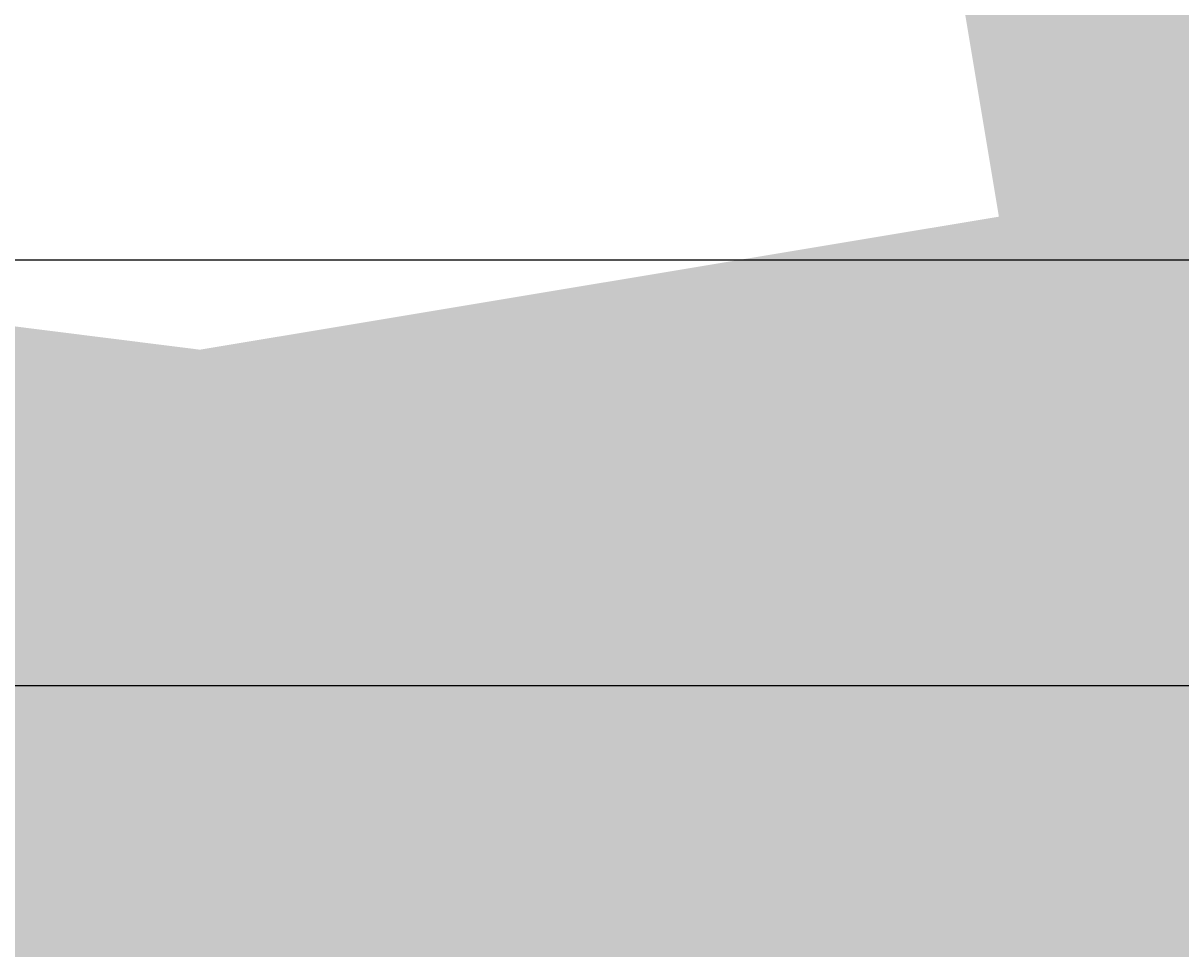
# Model space of a CAD drawing. Units: millimetres. Extents: x -22994 to 29398, y -19990 to 20176.
# Tile 120 of 135: x 245 to 296, y 124 to 165. Entities that reach past the tile are written whole.
import ezdxf

# ---------------------------------------------------------------- set-up
doc = ezdxf.new("R2010")
doc.units = ezdxf.units.MM
doc.header["$MEASUREMENT"] = 0
doc.layers.add('M-DIMS', color=2, linetype='Continuous', lineweight=18)
doc.styles.get("Standard").update_dxf_attribs({"font": 'arial.ttf'})
doc.dimstyles.get("Standard").update_dxf_attribs({"dimtxt": 0.18, "dimasz": 10000, "dimexe": 0.18, "dimexo": 0.0625, "dimgap": 0.09, "dimtad": 0, "dimtih": 1, "dimtoh": 1, "dimdec": 0, "dimzin": 0, "dimdsep": 46, "dimtxsty": 'Standard', "dimcen": 0.09, "dimadec": 0, "dimazin": 0, "dimtfac": 1, "dimtdec": 0, "dimtofl": 0, "dimtmove": 0, "dimatfit": 3, "dimfxl": 1, "dimtolj": 1, "dimtzin": 0, "dimlwd": 30, "dimarcsym": 0})

# ---------------------------------------------------------------- blocks, each defined once
blk = doc.blocks.new('*D2')
at = {"layer": 'Defpoints', "color": 0, "transparency": 16777216}
for p in [(6.677, 10.271), (290.852, 10.271), (290.852, -5.079)]:
    blk.add_point(p, dxfattribs=at)
at = {"layer": 'M-DIMS', "color": 0, "lineweight": -2, "transparency": 16777216}
for p, q in [((6.677, 10.209), (6.677, -5.259)), ((290.852, 10.209), (290.852, -5.259))]:
    blk.add_line(p, q, dxfattribs=at)
at = {"layer": 'M-DIMS', "color": 0, "lineweight": 30, "transparency": 16777216}
for p, q in [((-9993.323, -5.079), (-19993.323, -5.079)), ((10290.852, -5.079), (20290.852, -5.079))]:
    blk.add_line(p, q, dxfattribs=at)
at = {"layer": 'M-DIMS', "color": 0, "transparency": 16777216}
for points in [[(-9993.323, 1661.588), (-9993.323, -1671.745), (6.677, -5.079)], [(10290.852, 1661.588), (10290.852, -1671.745), (290.852, -5.079)]]:
    blk.add_solid(points, dxfattribs=at)
at = {"layer": 'M-DIMS', "color": 0, "transparency": 16777216, "insert": (148.765, -5.079), "char_height": 0.18, "attachment_point": 5}
blk.add_mtext('\\A1;284.2', dxfattribs=at)
blk = doc.blocks.new('*D3')
at = {"layer": 'Defpoints', "color": 0, "transparency": 16777216}
for p in [(110.265, 204.165), (110.265, 176.366), (95.833, 127.967)]:
    blk.add_point(p, dxfattribs=at)
at = {"layer": 'M-DIMS', "color": 0, "lineweight": 30, "transparency": 16777216}
for p, q in [((-9904.167, 204.165), (-19904.167, 204.165)), ((10110.265, 204.165), (20110.265, 204.165))]:
    blk.add_line(p, q, dxfattribs=at)
at = {"layer": 'M-DIMS', "color": 0, "lineweight": -2, "transparency": 16777216}
for p, q in [((95.833, 128.03), (95.833, 204.345)), ((110.265, 176.429), (110.265, 204.345))]:
    blk.add_line(p, q, dxfattribs=at)
at = {"layer": 'M-DIMS', "color": 0, "transparency": 16777216}
for points in [[(-9904.167, 1870.832), (-9904.167, -1462.501), (95.833, 204.165)], [(10110.265, 1870.832), (10110.265, -1462.501), (110.265, 204.165)]]:
    blk.add_solid(points, dxfattribs=at)
at = {"layer": 'M-DIMS', "color": 0, "transparency": 16777216, "insert": (103.049, 204.165), "char_height": 0.18, "attachment_point": 5}
blk.add_mtext('\\A1;14.432', dxfattribs=at)
blk = doc.blocks.new('*D4')
at = {"layer": 'Defpoints', "color": 0, "transparency": 16777216}
for p in [(116.265, 204.165), (110.265, 176.366), (116.265, 176.366)]:
    blk.add_point(p, dxfattribs=at)
at = {"layer": 'M-DIMS', "color": 0, "lineweight": 30, "transparency": 16777216}
for p, q in [((-9889.735, 204.165), (-19889.735, 204.165)), ((10116.265, 204.165), (20116.265, 204.165))]:
    blk.add_line(p, q, dxfattribs=at)
at = {"layer": 'M-DIMS', "color": 0, "lineweight": -2, "transparency": 16777216}
for p, q in [((110.265, 176.429), (110.265, 204.345)), ((116.265, 176.429), (116.265, 204.345))]:
    blk.add_line(p, q, dxfattribs=at)
at = {"layer": 'M-DIMS', "color": 0, "transparency": 16777216}
for points in [[(-9889.735, 1870.832), (-9889.735, -1462.501), (110.265, 204.165)], [(10116.265, 1870.832), (10116.265, -1462.501), (116.265, 204.165)]]:
    blk.add_solid(points, dxfattribs=at)
at = {"layer": 'M-DIMS', "color": 0, "transparency": 16777216, "insert": (113.265, 204.165), "char_height": 0.18, "attachment_point": 5}
blk.add_mtext('\\A1;6', dxfattribs=at)
blk = doc.blocks.new('*D5')
at = {"layer": 'Defpoints', "color": 0, "transparency": 16777216}
for p in [(181.265, 204.165), (116.265, 176.366), (181.265, 176.366)]:
    blk.add_point(p, dxfattribs=at)
at = {"layer": 'M-DIMS', "color": 0, "lineweight": 30, "transparency": 16777216}
for p, q in [((-9883.735, 204.165), (-19883.735, 204.165)), ((10181.265, 204.165), (20181.265, 204.165))]:
    blk.add_line(p, q, dxfattribs=at)
at = {"layer": 'M-DIMS', "color": 0, "lineweight": -2, "transparency": 16777216}
for p, q in [((116.265, 176.429), (116.265, 204.345)), ((181.265, 176.429), (181.265, 204.345))]:
    blk.add_line(p, q, dxfattribs=at)
at = {"layer": 'M-DIMS', "color": 0, "transparency": 16777216}
for points in [[(-9883.735, 1870.832), (-9883.735, -1462.501), (116.265, 204.165)], [(10181.265, 1870.832), (10181.265, -1462.501), (181.265, 204.165)]]:
    blk.add_solid(points, dxfattribs=at)
at = {"layer": 'M-DIMS', "color": 0, "transparency": 16777216, "insert": (148.765, 204.165), "char_height": 0.18, "attachment_point": 5}
blk.add_mtext('\\A1;65', dxfattribs=at)
blk = doc.blocks.new('*D6')
at = {"layer": 'Defpoints', "color": 0, "transparency": 16777216}
for p in [(187.265, 204.165), (181.265, 176.366), (187.265, 176.366)]:
    blk.add_point(p, dxfattribs=at)
at = {"layer": 'M-DIMS', "color": 0, "lineweight": 30, "transparency": 16777216}
for p, q in [((-9818.735, 204.165), (-19818.735, 204.165)), ((10187.265, 204.165), (20187.265, 204.165))]:
    blk.add_line(p, q, dxfattribs=at)
at = {"layer": 'M-DIMS', "color": 0, "lineweight": -2, "transparency": 16777216}
for p, q in [((181.265, 176.429), (181.265, 204.345)), ((187.265, 176.429), (187.265, 204.345))]:
    blk.add_line(p, q, dxfattribs=at)
at = {"layer": 'M-DIMS', "color": 0, "transparency": 16777216}
for points in [[(-9818.735, 1870.832), (-9818.735, -1462.501), (181.265, 204.165)], [(10187.265, 1870.832), (10187.265, -1462.501), (187.265, 204.165)]]:
    blk.add_solid(points, dxfattribs=at)
at = {"layer": 'M-DIMS', "color": 0, "transparency": 16777216, "insert": (184.265, 204.165), "char_height": 0.18, "attachment_point": 5}
blk.add_mtext('\\A1;6', dxfattribs=at)
blk = doc.blocks.new('*D7')
at = {"layer": 'Defpoints', "color": 0, "transparency": 16777216}
for p in [(201.697, 204.165), (187.265, 176.366), (201.697, 127.967)]:
    blk.add_point(p, dxfattribs=at)
at = {"layer": 'M-DIMS', "color": 0, "lineweight": 30, "transparency": 16777216}
for p, q in [((-9812.735, 204.165), (-19812.735, 204.165)), ((10201.697, 204.165), (20201.697, 204.165))]:
    blk.add_line(p, q, dxfattribs=at)
at = {"layer": 'M-DIMS', "color": 0, "lineweight": -2, "transparency": 16777216}
for p, q in [((187.265, 176.429), (187.265, 204.345)), ((201.697, 128.03), (201.697, 204.345))]:
    blk.add_line(p, q, dxfattribs=at)
at = {"layer": 'M-DIMS', "color": 0, "transparency": 16777216}
for points in [[(-9812.735, 1870.832), (-9812.735, -1462.501), (187.265, 204.165)], [(10201.697, 1870.832), (10201.697, -1462.501), (201.697, 204.165)]]:
    blk.add_solid(points, dxfattribs=at)
at = {"layer": 'M-DIMS', "color": 0, "transparency": 16777216, "insert": (194.481, 204.165), "char_height": 0.18, "attachment_point": 5}
blk.add_mtext('\\A1;14.432', dxfattribs=at)
blk = doc.blocks.new('*D8')
at = {"layer": 'Defpoints', "color": 0, "transparency": 16777216}
for p in [(227.648, 204.165), (227.648, 146.73), (201.697, 127.967)]:
    blk.add_point(p, dxfattribs=at)
at = {"layer": 'M-DIMS', "color": 0, "lineweight": 30, "transparency": 16777216}
for p, q in [((-9798.303, 204.165), (-19798.303, 204.165)), ((10227.648, 204.165), (20227.648, 204.165))]:
    blk.add_line(p, q, dxfattribs=at)
at = {"layer": 'M-DIMS', "color": 0, "lineweight": -2, "transparency": 16777216}
for p, q in [((201.697, 128.03), (201.697, 204.345)), ((227.648, 146.792), (227.648, 204.345))]:
    blk.add_line(p, q, dxfattribs=at)
at = {"layer": 'M-DIMS', "color": 0, "transparency": 16777216}
for points in [[(-9798.303, 1870.832), (-9798.303, -1462.501), (201.697, 204.165)], [(10227.648, 1870.832), (10227.648, -1462.501), (227.648, 204.165)]]:
    blk.add_solid(points, dxfattribs=at)
at = {"layer": 'M-DIMS', "color": 0, "transparency": 16777216, "insert": (214.673, 204.165), "char_height": 0.18, "attachment_point": 5}
blk.add_mtext('\\A1;25.95', dxfattribs=at)
blk = doc.blocks.new('*D9')
at = {"layer": 'Defpoints', "color": 0, "transparency": 16777216}
for p in [(187.265, 176.366), (306.202, 176.366), (290.852, 10.271)]:
    blk.add_point(p, dxfattribs=at)
at = {"layer": 'M-DIMS', "color": 0, "lineweight": 30, "transparency": 16777216}
for p, q in [((306.202, 10176.366), (306.202, 20176.366)), ((306.202, -9989.729), (306.202, -19989.729))]:
    blk.add_line(p, q, dxfattribs=at)
at = {"layer": 'M-DIMS', "color": 0, "lineweight": -2, "transparency": 16777216}
for p, q in [((187.327, 176.366), (306.382, 176.366)), ((290.915, 10.271), (306.382, 10.271))]:
    blk.add_line(p, q, dxfattribs=at)
at = {"layer": 'M-DIMS', "color": 0, "transparency": 16777216}
for points in [[(-1360.465, 10176.366), (1972.869, 10176.366), (306.202, 176.366)], [(-1360.465, -9989.729), (1972.869, -9989.729), (306.202, 10.271)]]:
    blk.add_solid(points, dxfattribs=at)
at = {"layer": 'M-DIMS', "color": 0, "transparency": 16777216, "insert": (306.202, 93.319), "char_height": 0.18, "attachment_point": 5}
blk.add_mtext('\\A1;166.1', dxfattribs=at)
blk = doc.blocks.new('*D10')
at = {"layer": 'Defpoints', "color": 0, "transparency": 16777216}
for p in [(125.65, 136.071), (133.346, 136.071), (133.346, -5.079)]:
    blk.add_point(p, dxfattribs=at)
at = {"layer": 'M-DIMS', "color": 0, "lineweight": -2, "transparency": 16777216}
for p, q in [((125.65, 136.009), (125.65, -5.259)), ((133.346, 136.009), (133.346, -5.259))]:
    blk.add_line(p, q, dxfattribs=at)
at = {"layer": 'M-DIMS', "color": 0, "lineweight": 30, "transparency": 16777216}
for p, q in [((-9874.35, -5.079), (-19874.35, -5.079)), ((10133.346, -5.079), (20133.346, -5.079))]:
    blk.add_line(p, q, dxfattribs=at)
at = {"layer": 'M-DIMS', "color": 0, "transparency": 16777216}
for points in [[(-9874.35, 1661.588), (-9874.35, -1671.745), (125.65, -5.079)], [(10133.346, 1661.588), (10133.346, -1671.745), (133.346, -5.079)]]:
    blk.add_solid(points, dxfattribs=at)
at = {"layer": 'M-DIMS', "color": 0, "transparency": 16777216, "insert": (129.498, -5.079), "char_height": 0.18, "attachment_point": 5}
blk.add_mtext('\\A1;7.696', dxfattribs=at)
blk = doc.blocks.new('*D11')
at = {"layer": 'Defpoints', "color": 0, "transparency": 16777216}
for p in [(133.346, 136.071), (135.65, 136.071), (135.65, -5.079)]:
    blk.add_point(p, dxfattribs=at)
at = {"layer": 'M-DIMS', "color": 0, "lineweight": -2, "transparency": 16777216}
for p, q in [((133.346, 136.009), (133.346, -5.259)), ((135.65, 136.009), (135.65, -5.259))]:
    blk.add_line(p, q, dxfattribs=at)
at = {"layer": 'M-DIMS', "color": 0, "lineweight": 30, "transparency": 16777216}
for p, q in [((-9866.654, -5.079), (-19866.654, -5.079)), ((10135.65, -5.079), (20135.65, -5.079))]:
    blk.add_line(p, q, dxfattribs=at)
at = {"layer": 'M-DIMS', "color": 0, "transparency": 16777216}
for points in [[(-9866.654, 1661.588), (-9866.654, -1671.745), (133.346, -5.079)], [(10135.65, 1661.588), (10135.65, -1671.745), (135.65, -5.079)]]:
    blk.add_solid(points, dxfattribs=at)
at = {"layer": 'M-DIMS', "color": 0, "transparency": 16777216, "insert": (134.498, -5.079), "char_height": 0.18, "attachment_point": 5}
blk.add_mtext('\\A1;2.304', dxfattribs=at)
blk = doc.blocks.new('*D12')
at = {"layer": 'Defpoints', "color": 0, "transparency": 16777216}
for p in [(135.65, 136.071), (145.65, 136.071), (145.65, -5.079)]:
    blk.add_point(p, dxfattribs=at)
at = {"layer": 'M-DIMS', "color": 0, "lineweight": -2, "transparency": 16777216}
for p, q in [((135.65, 136.009), (135.65, -5.259)), ((145.65, 136.009), (145.65, -5.259))]:
    blk.add_line(p, q, dxfattribs=at)
at = {"layer": 'M-DIMS', "color": 0, "lineweight": 30, "transparency": 16777216}
for p, q in [((-9864.35, -5.079), (-19864.35, -5.079)), ((10145.65, -5.079), (20145.65, -5.079))]:
    blk.add_line(p, q, dxfattribs=at)
at = {"layer": 'M-DIMS', "color": 0, "transparency": 16777216}
for points in [[(-9864.35, 1661.588), (-9864.35, -1671.745), (135.65, -5.079)], [(10145.65, 1661.588), (10145.65, -1671.745), (145.65, -5.079)]]:
    blk.add_solid(points, dxfattribs=at)
at = {"layer": 'M-DIMS', "color": 0, "transparency": 16777216, "insert": (140.65, -5.079), "char_height": 0.18, "attachment_point": 5}
blk.add_mtext('\\A1;10', dxfattribs=at)
blk = doc.blocks.new('*D13')
at = {"layer": 'Defpoints', "color": 0, "transparency": 16777216}
for p in [(145.65, 136.071), (155.65, 136.071), (155.65, -5.079)]:
    blk.add_point(p, dxfattribs=at)
at = {"layer": 'M-DIMS', "color": 0, "lineweight": -2, "transparency": 16777216}
for p, q in [((145.65, 136.009), (145.65, -5.259)), ((155.65, 136.009), (155.65, -5.259))]:
    blk.add_line(p, q, dxfattribs=at)
at = {"layer": 'M-DIMS', "color": 0, "lineweight": 30, "transparency": 16777216}
for p, q in [((-9854.35, -5.079), (-19854.35, -5.079)), ((10155.65, -5.079), (20155.65, -5.079))]:
    blk.add_line(p, q, dxfattribs=at)
at = {"layer": 'M-DIMS', "color": 0, "transparency": 16777216}
for points in [[(-9854.35, 1661.588), (-9854.35, -1671.745), (145.65, -5.079)], [(10155.65, 1661.588), (10155.65, -1671.745), (155.65, -5.079)]]:
    blk.add_solid(points, dxfattribs=at)
at = {"layer": 'M-DIMS', "color": 0, "transparency": 16777216, "insert": (150.65, -5.079), "char_height": 0.18, "attachment_point": 5}
blk.add_mtext('\\A1;10', dxfattribs=at)
blk = doc.blocks.new('*D14')
at = {"layer": 'Defpoints', "color": 0, "transparency": 16777216}
for p in [(155.65, 136.071), (165.65, 136.071), (165.65, -5.079)]:
    blk.add_point(p, dxfattribs=at)
at = {"layer": 'M-DIMS', "color": 0, "lineweight": -2, "transparency": 16777216}
for p, q in [((155.65, 136.009), (155.65, -5.259)), ((165.65, 136.009), (165.65, -5.259))]:
    blk.add_line(p, q, dxfattribs=at)
at = {"layer": 'M-DIMS', "color": 0, "lineweight": 30, "transparency": 16777216}
for p, q in [((-9844.35, -5.079), (-19844.35, -5.079)), ((10165.65, -5.079), (20165.65, -5.079))]:
    blk.add_line(p, q, dxfattribs=at)
at = {"layer": 'M-DIMS', "color": 0, "transparency": 16777216}
for points in [[(-9844.35, 1661.588), (-9844.35, -1671.745), (155.65, -5.079)], [(10165.65, 1661.588), (10165.65, -1671.745), (165.65, -5.079)]]:
    blk.add_solid(points, dxfattribs=at)
at = {"layer": 'M-DIMS', "color": 0, "transparency": 16777216, "insert": (160.65, -5.079), "char_height": 0.18, "attachment_point": 5}
blk.add_mtext('\\A1;10', dxfattribs=at)
blk = doc.blocks.new('*D15')
at = {"layer": 'Defpoints', "color": 0, "transparency": 16777216}
for p in [(173.346, 154.788), (173.346, 136.071), (306.202, 136.071)]:
    blk.add_point(p, dxfattribs=at)
at = {"layer": 'M-DIMS', "color": 0, "lineweight": 30, "transparency": 16777216}
for p, q in [((306.202, 10154.788), (306.202, 20154.788)), ((306.202, -9863.929), (306.202, -19863.929))]:
    blk.add_line(p, q, dxfattribs=at)
at = {"layer": 'M-DIMS', "color": 0, "lineweight": -2, "transparency": 16777216}
for p, q in [((173.408, 154.788), (306.382, 154.788)), ((173.408, 136.071), (306.382, 136.071))]:
    blk.add_line(p, q, dxfattribs=at)
at = {"layer": 'M-DIMS', "color": 0, "transparency": 16777216}
for points in [[(-1360.465, 10154.788), (1972.869, 10154.788), (306.202, 154.788)], [(-1360.465, -9863.929), (1972.869, -9863.929), (306.202, 136.071)]]:
    blk.add_solid(points, dxfattribs=at)
at = {"layer": 'M-DIMS', "color": 0, "transparency": 16777216, "insert": (306.202, 145.43), "char_height": 0.18, "attachment_point": 5}
blk.add_mtext('\\A1;18.717', dxfattribs=at)
blk = doc.blocks.new('*D16')
at = {"layer": 'Defpoints', "color": 0, "transparency": 16777216}
for p in [(120.17, 204.165), (110.466, 48.035), (120.17, 48.035)]:
    blk.add_point(p, dxfattribs=at)
at = {"layer": 'M-DIMS', "color": 0, "lineweight": 30, "transparency": 16777216}
for p, q in [((-9889.534, 204.165), (-19889.534, 204.165)), ((10120.17, 204.165), (20120.17, 204.165))]:
    blk.add_line(p, q, dxfattribs=at)
at = {"layer": 'M-DIMS', "color": 0, "lineweight": -2, "transparency": 16777216}
for p, q in [((110.466, 48.097), (110.466, 204.345)), ((120.17, 48.097), (120.17, 204.345))]:
    blk.add_line(p, q, dxfattribs=at)
at = {"layer": 'M-DIMS', "color": 0, "transparency": 16777216}
for points in [[(-9889.534, 1870.832), (-9889.534, -1462.501), (110.466, 204.165)], [(10120.17, 1870.832), (10120.17, -1462.501), (120.17, 204.165)]]:
    blk.add_solid(points, dxfattribs=at)
at = {"layer": 'M-DIMS', "color": 0, "transparency": 16777216, "insert": (115.318, 204.165), "char_height": 0.18, "attachment_point": 5}
blk.add_mtext('\\A1;9.704', dxfattribs=at)
blk = doc.blocks.new('*D17')
at = {"layer": 'Defpoints', "color": 0, "transparency": 16777216}
for p in [(126.17, 204.165), (120.17, 48.035), (126.17, 48.035)]:
    blk.add_point(p, dxfattribs=at)
at = {"layer": 'M-DIMS', "color": 0, "lineweight": 30, "transparency": 16777216}
for p, q in [((-9879.83, 204.165), (-19879.83, 204.165)), ((10126.17, 204.165), (20126.17, 204.165))]:
    blk.add_line(p, q, dxfattribs=at)
at = {"layer": 'M-DIMS', "color": 0, "lineweight": -2, "transparency": 16777216}
for p, q in [((120.17, 48.097), (120.17, 204.345)), ((126.17, 48.097), (126.17, 204.345))]:
    blk.add_line(p, q, dxfattribs=at)
at = {"layer": 'M-DIMS', "color": 0, "transparency": 16777216}
for points in [[(-9879.83, 1870.832), (-9879.83, -1462.501), (120.17, 204.165)], [(10126.17, 1870.832), (10126.17, -1462.501), (126.17, 204.165)]]:
    blk.add_solid(points, dxfattribs=at)
at = {"layer": 'M-DIMS', "color": 0, "transparency": 16777216, "insert": (123.17, 204.165), "char_height": 0.18, "attachment_point": 5}
blk.add_mtext('\\A1;6', dxfattribs=at)
blk = doc.blocks.new('*D18')
at = {"layer": 'Defpoints', "color": 0, "transparency": 16777216}
for p in [(132.17, 204.165), (126.17, 48.035), (132.17, 48.035)]:
    blk.add_point(p, dxfattribs=at)
at = {"layer": 'M-DIMS', "color": 0, "lineweight": 30, "transparency": 16777216}
for p, q in [((-9873.83, 204.165), (-19873.83, 204.165)), ((10132.17, 204.165), (20132.17, 204.165))]:
    blk.add_line(p, q, dxfattribs=at)
at = {"layer": 'M-DIMS', "color": 0, "lineweight": -2, "transparency": 16777216}
for p, q in [((126.17, 48.097), (126.17, 204.345)), ((132.17, 48.097), (132.17, 204.345))]:
    blk.add_line(p, q, dxfattribs=at)
at = {"layer": 'M-DIMS', "color": 0, "transparency": 16777216}
for points in [[(-9873.83, 1870.832), (-9873.83, -1462.501), (126.17, 204.165)], [(10132.17, 1870.832), (10132.17, -1462.501), (132.17, 204.165)]]:
    blk.add_solid(points, dxfattribs=at)
at = {"layer": 'M-DIMS', "color": 0, "transparency": 16777216, "insert": (129.17, 204.165), "char_height": 0.18, "attachment_point": 5}
blk.add_mtext('\\A1;6', dxfattribs=at)
blk = doc.blocks.new('*D19')
at = {"layer": 'Defpoints', "color": 0, "transparency": 16777216}
for p in [(138.17, 204.165), (132.17, 48.035), (138.17, 48.035)]:
    blk.add_point(p, dxfattribs=at)
at = {"layer": 'M-DIMS', "color": 0, "lineweight": 30, "transparency": 16777216}
for p, q in [((-9867.83, 204.165), (-19867.83, 204.165)), ((10138.17, 204.165), (20138.17, 204.165))]:
    blk.add_line(p, q, dxfattribs=at)
at = {"layer": 'M-DIMS', "color": 0, "lineweight": -2, "transparency": 16777216}
for p, q in [((132.17, 48.097), (132.17, 204.345)), ((138.17, 48.097), (138.17, 204.345))]:
    blk.add_line(p, q, dxfattribs=at)
at = {"layer": 'M-DIMS', "color": 0, "transparency": 16777216}
for points in [[(-9867.83, 1870.832), (-9867.83, -1462.501), (132.17, 204.165)], [(10138.17, 1870.832), (10138.17, -1462.501), (138.17, 204.165)]]:
    blk.add_solid(points, dxfattribs=at)
at = {"layer": 'M-DIMS', "color": 0, "transparency": 16777216, "insert": (135.17, 204.165), "char_height": 0.18, "attachment_point": 5}
blk.add_mtext('\\A1;6', dxfattribs=at)
blk = doc.blocks.new('*D20')
at = {"layer": 'Defpoints', "color": 0, "transparency": 16777216}
for p in [(144.17, 204.165), (138.17, 48.035), (144.17, 48.035)]:
    blk.add_point(p, dxfattribs=at)
at = {"layer": 'M-DIMS', "color": 0, "lineweight": 30, "transparency": 16777216}
for p, q in [((-9861.83, 204.165), (-19861.83, 204.165)), ((10144.17, 204.165), (20144.17, 204.165))]:
    blk.add_line(p, q, dxfattribs=at)
at = {"layer": 'M-DIMS', "color": 0, "lineweight": -2, "transparency": 16777216}
for p, q in [((138.17, 48.097), (138.17, 204.345)), ((144.17, 48.097), (144.17, 204.345))]:
    blk.add_line(p, q, dxfattribs=at)
at = {"layer": 'M-DIMS', "color": 0, "transparency": 16777216}
for points in [[(-9861.83, 1870.832), (-9861.83, -1462.501), (138.17, 204.165)], [(10144.17, 1870.832), (10144.17, -1462.501), (144.17, 204.165)]]:
    blk.add_solid(points, dxfattribs=at)
at = {"layer": 'M-DIMS', "color": 0, "transparency": 16777216, "insert": (141.17, 204.165), "char_height": 0.18, "attachment_point": 5}
blk.add_mtext('\\A1;6', dxfattribs=at)
blk = doc.blocks.new('*D21')
at = {"layer": 'Defpoints', "color": 0, "transparency": 16777216}
for p in [(149.116, 204.165), (144.17, 48.035), (149.116, 48.035)]:
    blk.add_point(p, dxfattribs=at)
at = {"layer": 'M-DIMS', "color": 0, "lineweight": 30, "transparency": 16777216}
for p, q in [((-9855.83, 204.165), (-19855.83, 204.165)), ((10149.116, 204.165), (20149.116, 204.165))]:
    blk.add_line(p, q, dxfattribs=at)
at = {"layer": 'M-DIMS', "color": 0, "lineweight": -2, "transparency": 16777216}
for p, q in [((144.17, 48.097), (144.17, 204.345)), ((149.116, 48.097), (149.116, 204.345))]:
    blk.add_line(p, q, dxfattribs=at)
at = {"layer": 'M-DIMS', "color": 0, "transparency": 16777216}
for points in [[(-9855.83, 1870.832), (-9855.83, -1462.501), (144.17, 204.165)], [(10149.116, 1870.832), (10149.116, -1462.501), (149.116, 204.165)]]:
    blk.add_solid(points, dxfattribs=at)
at = {"layer": 'M-DIMS', "color": 0, "transparency": 16777216, "insert": (146.643, 204.165), "char_height": 0.18, "attachment_point": 5}
blk.add_mtext('\\A1;4.945', dxfattribs=at)
blk = doc.blocks.new('*D22')
at = {"layer": 'Defpoints', "color": 0, "transparency": 16777216}
for p in [(149.116, 30.99), (155.116, 30.99), (155.116, -5.079)]:
    blk.add_point(p, dxfattribs=at)
at = {"layer": 'M-DIMS', "color": 0, "lineweight": -2, "transparency": 16777216}
for p, q in [((149.116, 30.927), (149.116, -5.259)), ((155.116, 30.927), (155.116, -5.259))]:
    blk.add_line(p, q, dxfattribs=at)
at = {"layer": 'M-DIMS', "color": 0, "lineweight": 30, "transparency": 16777216}
for p, q in [((-9850.884, -5.079), (-19850.884, -5.079)), ((10155.116, -5.079), (20155.116, -5.079))]:
    blk.add_line(p, q, dxfattribs=at)
at = {"layer": 'M-DIMS', "color": 0, "transparency": 16777216}
for points in [[(-9850.884, 1661.588), (-9850.884, -1671.745), (149.116, -5.079)], [(10155.116, 1661.588), (10155.116, -1671.745), (155.116, -5.079)]]:
    blk.add_solid(points, dxfattribs=at)
at = {"layer": 'M-DIMS', "color": 0, "transparency": 16777216, "insert": (152.116, -5.079), "char_height": 0.18, "attachment_point": 5}
blk.add_mtext('\\A1;6', dxfattribs=at)
blk = doc.blocks.new('*D23')
at = {"layer": 'Defpoints', "color": 0, "transparency": 16777216}
for p in [(155.116, 30.99), (161.116, 30.99), (161.116, -5.079)]:
    blk.add_point(p, dxfattribs=at)
at = {"layer": 'M-DIMS', "color": 0, "lineweight": -2, "transparency": 16777216}
for p, q in [((155.116, 30.927), (155.116, -5.259)), ((161.116, 30.927), (161.116, -5.259))]:
    blk.add_line(p, q, dxfattribs=at)
at = {"layer": 'M-DIMS', "color": 0, "lineweight": 30, "transparency": 16777216}
for p, q in [((-9844.884, -5.079), (-19844.884, -5.079)), ((10161.116, -5.079), (20161.116, -5.079))]:
    blk.add_line(p, q, dxfattribs=at)
at = {"layer": 'M-DIMS', "color": 0, "transparency": 16777216}
for points in [[(-9844.884, 1661.588), (-9844.884, -1671.745), (155.116, -5.079)], [(10161.116, 1661.588), (10161.116, -1671.745), (161.116, -5.079)]]:
    blk.add_solid(points, dxfattribs=at)
at = {"layer": 'M-DIMS', "color": 0, "transparency": 16777216, "insert": (158.116, -5.079), "char_height": 0.18, "attachment_point": 5}
blk.add_mtext('\\A1;6', dxfattribs=at)
blk = doc.blocks.new('*D24')
at = {"layer": 'Defpoints', "color": 0, "transparency": 16777216}
for p in [(161.116, 30.99), (166.439, 30.99), (166.439, -5.079)]:
    blk.add_point(p, dxfattribs=at)
at = {"layer": 'M-DIMS', "color": 0, "lineweight": -2, "transparency": 16777216}
for p, q in [((161.116, 30.927), (161.116, -5.259)), ((166.439, 30.927), (166.439, -5.259))]:
    blk.add_line(p, q, dxfattribs=at)
at = {"layer": 'M-DIMS', "color": 0, "lineweight": 30, "transparency": 16777216}
for p, q in [((-9838.884, -5.079), (-19838.884, -5.079)), ((10166.439, -5.079), (20166.439, -5.079))]:
    blk.add_line(p, q, dxfattribs=at)
at = {"layer": 'M-DIMS', "color": 0, "transparency": 16777216}
for points in [[(-9838.884, 1661.588), (-9838.884, -1671.745), (161.116, -5.079)], [(10166.439, 1661.588), (10166.439, -1671.745), (166.439, -5.079)]]:
    blk.add_solid(points, dxfattribs=at)
at = {"layer": 'M-DIMS', "color": 0, "transparency": 16777216, "insert": (163.777, -5.079), "char_height": 0.18, "attachment_point": 5}
blk.add_mtext('\\A1;5.323', dxfattribs=at)
blk = doc.blocks.new('*D25')
at = {"layer": 'Defpoints', "color": 0, "transparency": 16777216}
for p in [(166.439, 30.99), (172.439, 30.99), (172.439, -5.079)]:
    blk.add_point(p, dxfattribs=at)
at = {"layer": 'M-DIMS', "color": 0, "lineweight": -2, "transparency": 16777216}
for p, q in [((166.439, 30.927), (166.439, -5.259)), ((172.439, 30.927), (172.439, -5.259))]:
    blk.add_line(p, q, dxfattribs=at)
at = {"layer": 'M-DIMS', "color": 0, "lineweight": 30, "transparency": 16777216}
for p, q in [((-9833.561, -5.079), (-19833.561, -5.079)), ((10172.439, -5.079), (20172.439, -5.079))]:
    blk.add_line(p, q, dxfattribs=at)
at = {"layer": 'M-DIMS', "color": 0, "transparency": 16777216}
for points in [[(-9833.561, 1661.588), (-9833.561, -1671.745), (166.439, -5.079)], [(10172.439, 1661.588), (10172.439, -1671.745), (172.439, -5.079)]]:
    blk.add_solid(points, dxfattribs=at)
at = {"layer": 'M-DIMS', "color": 0, "transparency": 16777216, "insert": (169.439, -5.079), "char_height": 0.18, "attachment_point": 5}
blk.add_mtext('\\A1;6', dxfattribs=at)
blk = doc.blocks.new('*D26')
at = {"layer": 'Defpoints', "color": 0, "transparency": 16777216}
for p in [(172.439, 30.99), (178.439, 30.99), (178.439, -5.079)]:
    blk.add_point(p, dxfattribs=at)
at = {"layer": 'M-DIMS', "color": 0, "lineweight": -2, "transparency": 16777216}
for p, q in [((172.439, 30.927), (172.439, -5.259)), ((178.439, 30.927), (178.439, -5.259))]:
    blk.add_line(p, q, dxfattribs=at)
at = {"layer": 'M-DIMS', "color": 0, "lineweight": 30, "transparency": 16777216}
for p, q in [((-9827.561, -5.079), (-19827.561, -5.079)), ((10178.439, -5.079), (20178.439, -5.079))]:
    blk.add_line(p, q, dxfattribs=at)
at = {"layer": 'M-DIMS', "color": 0, "transparency": 16777216}
for points in [[(-9827.561, 1661.588), (-9827.561, -1671.745), (172.439, -5.079)], [(10178.439, 1661.588), (10178.439, -1671.745), (178.439, -5.079)]]:
    blk.add_solid(points, dxfattribs=at)
at = {"layer": 'M-DIMS', "color": 0, "transparency": 16777216, "insert": (175.439, -5.079), "char_height": 0.18, "attachment_point": 5}
blk.add_mtext('\\A1;6', dxfattribs=at)
blk = doc.blocks.new('*D27')
at = {"layer": 'Defpoints', "color": 0, "transparency": 16777216}
for p in [(178.439, 30.99), (188.117, 30.99), (188.117, -5.079)]:
    blk.add_point(p, dxfattribs=at)
at = {"layer": 'M-DIMS', "color": 0, "lineweight": -2, "transparency": 16777216}
for p, q in [((178.439, 30.927), (178.439, -5.259)), ((188.117, 30.927), (188.117, -5.259))]:
    blk.add_line(p, q, dxfattribs=at)
at = {"layer": 'M-DIMS', "color": 0, "lineweight": 30, "transparency": 16777216}
for p, q in [((-9821.561, -5.079), (-19821.561, -5.079)), ((10188.117, -5.079), (20188.117, -5.079))]:
    blk.add_line(p, q, dxfattribs=at)
at = {"layer": 'M-DIMS', "color": 0, "transparency": 16777216}
for points in [[(-9821.561, 1661.588), (-9821.561, -1671.745), (178.439, -5.079)], [(10188.117, 1661.588), (10188.117, -1671.745), (188.117, -5.079)]]:
    blk.add_solid(points, dxfattribs=at)
at = {"layer": 'M-DIMS', "color": 0, "transparency": 16777216, "insert": (183.278, -5.079), "char_height": 0.18, "attachment_point": 5}
blk.add_mtext('\\A1;9.679', dxfattribs=at)
blk = doc.blocks.new('*D28')
at = {"layer": 'Defpoints', "color": 0, "transparency": 16777216}
for p in [(188.117, 48.035), (306.202, 48.035), (188.117, 30.99)]:
    blk.add_point(p, dxfattribs=at)
at = {"layer": 'M-DIMS', "color": 0, "lineweight": 30, "transparency": 16777216}
for p, q in [((306.202, 10048.035), (306.202, 20048.035)), ((306.202, -9969.01), (306.202, -19969.01))]:
    blk.add_line(p, q, dxfattribs=at)
at = {"layer": 'M-DIMS', "color": 0, "lineweight": -2, "transparency": 16777216}
for p, q in [((188.18, 48.035), (306.382, 48.035)), ((188.18, 30.99), (306.382, 30.99))]:
    blk.add_line(p, q, dxfattribs=at)
at = {"layer": 'M-DIMS', "color": 0, "transparency": 16777216}
for points in [[(-1360.465, 10048.035), (1972.869, 10048.035), (306.202, 48.035)], [(-1360.465, -9969.01), (1972.869, -9969.01), (306.202, 30.99)]]:
    blk.add_solid(points, dxfattribs=at)
at = {"layer": 'M-DIMS', "color": 0, "transparency": 16777216, "insert": (306.202, 39.512), "char_height": 0.18, "attachment_point": 5}
blk.add_mtext('\\A1;17.045', dxfattribs=at)
blk = doc.blocks.new('*D29')
at = {"layer": 'Defpoints', "color": 0, "transparency": 16777216}
for p in [(36.801, 80.045), (64.03, 80.045)]:
    blk.add_point(p, dxfattribs=at)
at = {"layer": 'M-DIMS', "color": 0, "lineweight": -2, "transparency": 16777216}
for p, q in [((50.325, 80.045), (50.505, 80.045)), ((50.415, 79.955), (50.415, 80.135))]:
    blk.add_line(p, q, dxfattribs=at)
at = {"layer": 'M-DIMS', "color": 0, "lineweight": 30, "transparency": 16777216}
blk.add_line((20064.03, 80.03), (10064.03, 80.038), dxfattribs=at)
at = {"layer": 'M-DIMS', "color": 0, "transparency": 16777216}
blk.add_solid([(10064.031, 1746.704), (10064.028, -1586.629), (64.03, 80.045)], dxfattribs=at)
at = {"layer": 'M-DIMS', "color": 0, "transparency": 16777216, "insert": (20064.521, 80.03), "char_height": 0.18, "attachment_point": 5}
blk.add_mtext('\\A1;∅27.23', dxfattribs=at)
blk = doc.blocks.new('*D30')
at = {"layer": 'Defpoints', "color": 0, "transparency": 16777216}
for p in [(216.315, 146.729), (238.982, 146.73)]:
    blk.add_point(p, dxfattribs=at)
at = {"layer": 'M-DIMS', "color": 0, "lineweight": 30, "transparency": 16777216}
blk.add_line((20238.982, 147.496), (10238.982, 147.113), dxfattribs=at)
at = {"layer": 'M-DIMS', "color": 0, "lineweight": -2, "transparency": 16777216}
for p, q in [((227.558, 146.73), (227.738, 146.73)), ((227.648, 146.64), (227.648, 146.82))]:
    blk.add_line(p, q, dxfattribs=at)
at = {"layer": 'M-DIMS', "color": 0, "transparency": 16777216}
blk.add_solid([(10238.918, 1813.78), (10239.046, -1519.554), (238.982, 146.73)], dxfattribs=at)
at = {"layer": 'M-DIMS', "color": 0, "transparency": 16777216, "insert": (20239.544, 147.496), "char_height": 0.18, "attachment_point": 5}
blk.add_mtext('\\A1;∅22.667', dxfattribs=at)
blk = doc.blocks.new('*D31')
at = {"layer": 'Defpoints', "color": 0, "transparency": 16777216}
for p in [(223.164, 146.729), (232.133, 146.73)]:
    blk.add_point(p, dxfattribs=at)
at = {"layer": 'M-DIMS', "color": 0, "lineweight": 30, "transparency": 16777216}
blk.add_line((20232.133, 148.666), (10232.133, 147.698), dxfattribs=at)
at = {"layer": 'M-DIMS', "color": 0, "lineweight": -2, "transparency": 16777216}
for p, q in [((227.558, 146.73), (227.738, 146.73)), ((227.648, 146.64), (227.648, 146.82))]:
    blk.add_line(p, q, dxfattribs=at)
at = {"layer": 'M-DIMS', "color": 0, "transparency": 16777216}
blk.add_solid([(10231.971, 1814.364), (10232.294, -1518.969), (232.133, 146.73)], dxfattribs=at)
at = {"layer": 'M-DIMS', "color": 0, "transparency": 16777216, "insert": (20232.625, 148.666), "char_height": 0.18, "attachment_point": 5}
blk.add_mtext('\\A1;∅8.969', dxfattribs=at)
blk = doc.blocks.new('*D33')
at = {"layer": 'Defpoints', "color": 0, "transparency": 16777216}
for p in [(229.561, 154.377), (232.997, 153.351)]:
    blk.add_point(p, dxfattribs=at)
at = {"layer": 'M-DIMS', "color": 0, "lineweight": -2, "transparency": 16777216}
for p, q in [((229.471, 154.377), (229.651, 154.377)), ((229.561, 154.287), (229.561, 154.467))]:
    blk.add_line(p, q, dxfattribs=at)
at = {"layer": 'M-DIMS', "color": 0, "lineweight": 30, "transparency": 16777216}
for p, q in [((19396.339, -5570.838), (9814.668, -2708.743)), ((29396.339, -5570.838), (19396.339, -5570.838))]:
    blk.add_line(p, q, dxfattribs=at)
at = {"layer": 'M-DIMS', "color": 0, "transparency": 16777216}
blk.add_solid([(10291.684, -1111.798), (9337.652, -4305.689), (232.997, 153.351)], dxfattribs=at)
at = {"layer": 'M-DIMS', "color": 0, "transparency": 16777216, "insert": (29397.012, -5570.838), "char_height": 0.18, "attachment_point": 5}
blk.add_mtext('\\A1;6X R3.586', dxfattribs=at)
blk = doc.blocks.new('*D34')
at = {"layer": 'Defpoints', "color": 0, "transparency": 16777216}
for p in [(178.58, 122.895), (176.812, 121.128)]:
    blk.add_point(p, dxfattribs=at)
at = {"layer": 'M-DIMS', "color": 0, "lineweight": 30, "transparency": 16777216}
for p, q in [((14322.436, 14263.311), (7250.508, 7193.103)), ((24322.436, 14263.311), (14322.436, 14263.311))]:
    blk.add_line(p, q, dxfattribs=at)
at = {"layer": 'M-DIMS', "color": 0, "lineweight": -2, "transparency": 16777216}
for p, q in [((176.722, 121.128), (176.902, 121.128)), ((176.812, 121.038), (176.812, 121.218))]:
    blk.add_line(p, q, dxfattribs=at)
at = {"layer": 'M-DIMS', "color": 0, "transparency": 16777216}
blk.add_solid([(6072.14, 8371.758), (8428.876, 6014.448), (178.58, 122.895)], dxfattribs=at)
at = {"layer": 'M-DIMS', "color": 0, "transparency": 16777216, "insert": (24322.97, 14263.311), "char_height": 0.18, "attachment_point": 5}
blk.add_mtext('\\A1;6X R2.5', dxfattribs=at)
blk = doc.blocks.new('*D36')
at = {"layer": 'Defpoints', "color": 0, "transparency": 16777216}
for p in [(46.39, 31.303), (46.387, 26.593)]:
    blk.add_point(p, dxfattribs=at)
at = {"layer": 'M-DIMS', "color": 0, "lineweight": 30, "transparency": 16777216}
for p, q in [((57.15, 20031.301), (51.77, 10031.302)), ((10057.15, 20031.301), (57.15, 20031.301))]:
    blk.add_line(p, q, dxfattribs=at)
at = {"layer": 'M-DIMS', "color": 0, "lineweight": -2, "transparency": 16777216}
for p, q in [((46.389, 28.858), (46.389, 29.038)), ((46.299, 28.948), (46.479, 28.948))]:
    blk.add_line(p, q, dxfattribs=at)
at = {"layer": 'M-DIMS', "color": 0, "transparency": 16777216}
blk.add_solid([(-1614.896, 10032.199), (1718.436, 10030.405), (46.39, 31.303)], dxfattribs=at)
at = {"layer": 'M-DIMS', "color": 0, "transparency": 16777216, "insert": (10057.554, 20031.301), "char_height": 0.18, "attachment_point": 5}
blk.add_mtext('\\A1;∅4.71', dxfattribs=at)
blk = doc.blocks.new('*D37')
at = {"layer": 'Defpoints', "color": 0, "transparency": 16777216}
for p in [(54.834, 118.615), (59.494, 118.614)]:
    blk.add_point(p, dxfattribs=at)
at = {"layer": 'M-DIMS', "color": 0, "lineweight": -2, "transparency": 16777216}
for p, q in [((57.074, 118.614), (57.254, 118.614)), ((57.164, 118.524), (57.164, 118.704))]:
    blk.add_line(p, q, dxfattribs=at)
at = {"layer": 'M-DIMS', "color": 0, "lineweight": 30, "transparency": 16777216}
blk.add_line((20059.493, 116.253), (10059.494, 117.434), dxfattribs=at)
at = {"layer": 'M-DIMS', "color": 0, "transparency": 16777216}
blk.add_solid([(10059.69, 1784.1), (10059.297, -1549.233), (59.494, 118.614)], dxfattribs=at)
at = {"layer": 'M-DIMS', "color": 0, "transparency": 16777216, "insert": (20059.985, 116.253), "char_height": 0.18, "attachment_point": 5}
blk.add_mtext('\\A1;∅4.659', dxfattribs=at)

msp = doc.modelspace()

# ---------------------------------------------------------------- dimensions: what is measured, and where the dimension line sits
at = {"layer": 'M-DIMS'}
for base, p1, p2, override, picture, middle in [((306.202, 176.3662), (290.852, 10.2713), (187.2647, 176.3662), {"dimdec": 1, "dimlfac": 1, "dimrnd": 0, "dimzin": 0, "dimdsep": 46, "dimlunit": 2}, '*D9', (306.202, 93.3187)), ((306.202, 136.0713), (173.3459, 154.788), (173.3459, 136.0713), {"dimdec": 3, "dimlfac": 1, "dimrnd": 0, "dimzin": 0, "dimdsep": 46, "dimlunit": 2}, '*D15', (306.202, 145.4297)), ((306.202, 48.0349), (188.1175, 30.9895), (188.1175, 48.0349), {"dimdec": 3, "dimlfac": 1, "dimrnd": 0, "dimzin": 0, "dimdsep": 46, "dimlunit": 2}, '*D28', (306.202, 39.5122))]:
    dim = msp.add_linear_dim(base=base, p1=p1, p2=p2, angle=90, dimstyle='Standard', override=override, dxfattribs=at)
    dim.commit()
    dim.dimension.update_dxf_attribs({"geometry": picture, "text_midpoint": middle})
for p1, p2, override, picture, middle in [((46.3875, 26.5934), (46.39, 31.3035), {"dimdec": 2, "dimlfac": 1, "dimrnd": 0, "dimzin": 0, "dimdsep": 46, "dimlunit": 2}, '*D36', (10057.5542, 20031.3006)), ((223.1641, 146.7291), (232.1328, 146.73), {"dimdec": 3, "dimlfac": 1, "dimrnd": 0, "dimzin": 0, "dimdsep": 46, "dimlunit": 2}, '*D31', (20232.1327, 148.6656)), ((216.3148, 146.7291), (238.9821, 146.73), {"dimdec": 3, "dimlfac": 1, "dimrnd": 0, "dimzin": 0, "dimdsep": 46, "dimlunit": 2}, '*D30', (20238.9821, 147.4959))]:
    dim = msp.add_diameter_dim_2p(p1=p1, p2=p2, dimstyle='Standard', override=override, dxfattribs=at)
    dim.commit()
    dim.dimension.update_dxf_attribs({"geometry": picture, "text_midpoint": middle, "dimtype": 163})
for center, mpoint, override, picture, middle in [((176.8123, 121.1277), (178.5802, 122.8952), {"dimdec": 1, "dimlfac": 1, "dimrnd": 0, "dimzin": 0, "dimdsep": 46, "dimlunit": 2}, '*D34', (24322.9703, 14263.3108)), ((229.5613, 154.3773), (232.9972, 153.3509), {"dimdec": 3, "dimlfac": 1, "dimrnd": 0, "dimzin": 0, "dimdsep": 46, "dimlunit": 2}, '*D33', (29397.0125, -5570.8378))]:
    dim = msp.add_radius_dim(center=center, mpoint=mpoint, text='6X <>', dimstyle='Standard', override=override, dxfattribs=at)
    dim.commit()
    dim.dimension.update_dxf_attribs({"geometry": picture, "text_midpoint": middle})
for base, p1, p2, override, picture, middle in [((110.2647, 204.1654), (95.8327, 127.967), (110.2647, 176.3662), {"dimdec": 3, "dimlfac": 1, "dimrnd": 0, "dimzin": 0, "dimdsep": 46, "dimlunit": 2}, '*D3', (103.0487, 204.1654)), ((116.2647, 204.1654), (110.2647, 176.3662), (116.2647, 176.3662), {"dimdec": 0, "dimlfac": 1, "dimrnd": 0, "dimzin": 0, "dimdsep": 46, "dimlunit": 2}, '*D4', (113.2647, 204.1654)), ((120.1702, 204.1654), (110.4658, 48.0349), (120.1702, 48.0349), {"dimdec": 3, "dimlfac": 1, "dimrnd": 0, "dimzin": 0, "dimdsep": 46, "dimlunit": 2}, '*D16', (115.318, 204.1654)), ((181.2647, 204.1654), (116.2647, 176.3662), (181.2647, 176.3662), {"dimdec": 0, "dimlfac": 1, "dimrnd": 0, "dimzin": 0, "dimdsep": 46, "dimlunit": 2}, '*D5', (148.7647, 204.1654)), ((126.1702, 204.1654), (120.1702, 48.0349), (126.1702, 48.0349), {"dimdec": 0, "dimlfac": 1, "dimrnd": 0, "dimzin": 0, "dimdsep": 46, "dimlunit": 2}, '*D17', (123.1702, 204.1654)), ((132.1702, 204.1654), (126.1702, 48.0349), (132.1702, 48.0349), {"dimdec": 0, "dimlfac": 1, "dimrnd": 0, "dimzin": 0, "dimdsep": 46, "dimlunit": 2}, '*D18', (129.1702, 204.1654)), ((138.1702, 204.1654), (132.1702, 48.0349), (138.1702, 48.0349), {"dimdec": 0, "dimlfac": 1, "dimrnd": 0, "dimzin": 0, "dimdsep": 46, "dimlunit": 2}, '*D19', (135.1702, 204.1654)), ((144.1702, 204.1654), (138.1702, 48.0349), (144.1702, 48.0349), {"dimdec": 0, "dimlfac": 1, "dimrnd": 0, "dimzin": 0, "dimdsep": 46, "dimlunit": 2}, '*D20', (141.1702, 204.1654)), ((149.11567, 204.16539), (144.17023, 48.03494), (149.11567, 48.03494), {"dimdec": 3, "dimlfac": 1, "dimrnd": 0, "dimzin": 0, "dimdsep": 46, "dimlunit": 2}, '*D21', (146.64295, 204.16539)), ((187.2647, 204.1654), (181.2647, 176.3662), (187.2647, 176.3662), {"dimdec": 0, "dimlfac": 1, "dimrnd": 0, "dimzin": 0, "dimdsep": 46, "dimlunit": 2}, '*D6', (184.2647, 204.1654)), ((201.6967, 204.1654), (187.2647, 176.3662), (201.6967, 127.967), {"dimdec": 3, "dimlfac": 1, "dimrnd": 0, "dimzin": 0, "dimdsep": 46, "dimlunit": 2}, '*D7', (194.4807, 204.1654)), ((227.6485, 204.1654), (201.6967, 127.967), (227.6485, 146.7296), {"dimdec": 2, "dimlfac": 1, "dimrnd": 0, "dimzin": 0, "dimdsep": 46, "dimlunit": 2}, '*D8', (214.6726, 204.1654)), ((290.852, -5.0787), (6.6773, 10.2713), (290.852, 10.2713), {"dimdec": 1, "dimlfac": 1, "dimrnd": 0, "dimzin": 0, "dimdsep": 46, "dimlunit": 2}, '*D2', (148.7647, -5.0787)), ((133.3459, -5.0787), (125.6498, 136.0713), (133.3459, 136.0713), {"dimdec": 3, "dimlfac": 1, "dimrnd": 0, "dimzin": 0, "dimdsep": 46, "dimlunit": 2}, '*D10', (129.4978, -5.0787)), ((135.6498, -5.0787), (133.3459, 136.0713), (135.6498, 136.0713), {"dimdec": 3, "dimlfac": 1, "dimrnd": 0, "dimzin": 0, "dimdsep": 46, "dimlunit": 2}, '*D11', (134.4978, -5.0787)), ((145.6498, -5.0787), (135.6498, 136.0713), (145.6498, 136.0713), {"dimdec": 0, "dimlfac": 1, "dimrnd": 0, "dimzin": 0, "dimdsep": 46, "dimlunit": 2}, '*D12', (140.6498, -5.0787)), ((155.6498, -5.0787), (145.6498, 136.0713), (155.6498, 136.0713), {"dimdec": 0, "dimlfac": 1, "dimrnd": 0, "dimzin": 0, "dimdsep": 46, "dimlunit": 2}, '*D13', (150.6498, -5.0787)), ((155.1157, -5.0787), (149.1157, 30.9895), (155.1157, 30.9895), {"dimdec": 0, "dimlfac": 1, "dimrnd": 0, "dimzin": 0, "dimdsep": 46, "dimlunit": 2}, '*D22', (152.1157, -5.0787)), ((161.1157, -5.0787), (155.1157, 30.9895), (161.1157, 30.9895), {"dimdec": 0, "dimlfac": 1, "dimrnd": 0, "dimzin": 0, "dimdsep": 46, "dimlunit": 2}, '*D23', (158.1157, -5.0787)), ((165.6498, -5.0787), (155.6498, 136.0713), (165.6498, 136.0713), {"dimdec": 0, "dimlfac": 1, "dimrnd": 0, "dimzin": 0, "dimdsep": 46, "dimlunit": 2}, '*D14', (160.6498, -5.0787)), ((166.4387, -5.0787), (161.1157, 30.9895), (166.4387, 30.9895), {"dimdec": 3, "dimlfac": 1, "dimrnd": 0, "dimzin": 0, "dimdsep": 46, "dimlunit": 2}, '*D24', (163.7772, -5.0787)), ((172.4387, -5.0787), (166.4387, 30.9895), (172.4387, 30.9895), {"dimdec": 0, "dimlfac": 1, "dimrnd": 0, "dimzin": 0, "dimdsep": 46, "dimlunit": 2}, '*D25', (169.4387, -5.0787)), ((178.4387, -5.0787), (172.4387, 30.9895), (178.4387, 30.9895), {"dimdec": 0, "dimlfac": 1, "dimrnd": 0, "dimzin": 0, "dimdsep": 46, "dimlunit": 2}, '*D26', (175.4387, -5.0787)), ((188.1175, -5.0787), (178.4387, 30.9895), (188.1175, 30.9895), {"dimdec": 3, "dimlfac": 1, "dimrnd": 0, "dimzin": 0, "dimdsep": 46, "dimlunit": 2}, '*D27', (183.2781, -5.0787))]:
    dim = msp.add_linear_dim(base=base, p1=p1, p2=p2, dimstyle='Standard', override=override, dxfattribs=at)
    dim.commit()
    dim.dimension.update_dxf_attribs({"geometry": picture, "text_midpoint": middle})
for p1, p2, override, picture, middle in [((54.8343, 118.6145), (59.4936, 118.614), {"dimdec": 3, "dimlfac": 1, "dimrnd": 0, "dimzin": 0, "dimdsep": 46, "dimlunit": 2}, '*D37', (20059.4934, 116.2531)), ((36.8006, 80.045), (64.0296, 80.045), {"dimdec": 2, "dimlfac": 1, "dimrnd": 0, "dimzin": 0, "dimdsep": 46, "dimlunit": 2}, '*D29', (20064.0296, 80.0303))]:
    dim = msp.add_diameter_dim_2p(p1=p1, p2=p2, dimstyle='Standard', override=override, dxfattribs=at)
    dim.commit()
    dim.dimension.update_dxf_attribs({"geometry": picture, "text_midpoint": middle})

doc.saveas('drawing.dxf')
